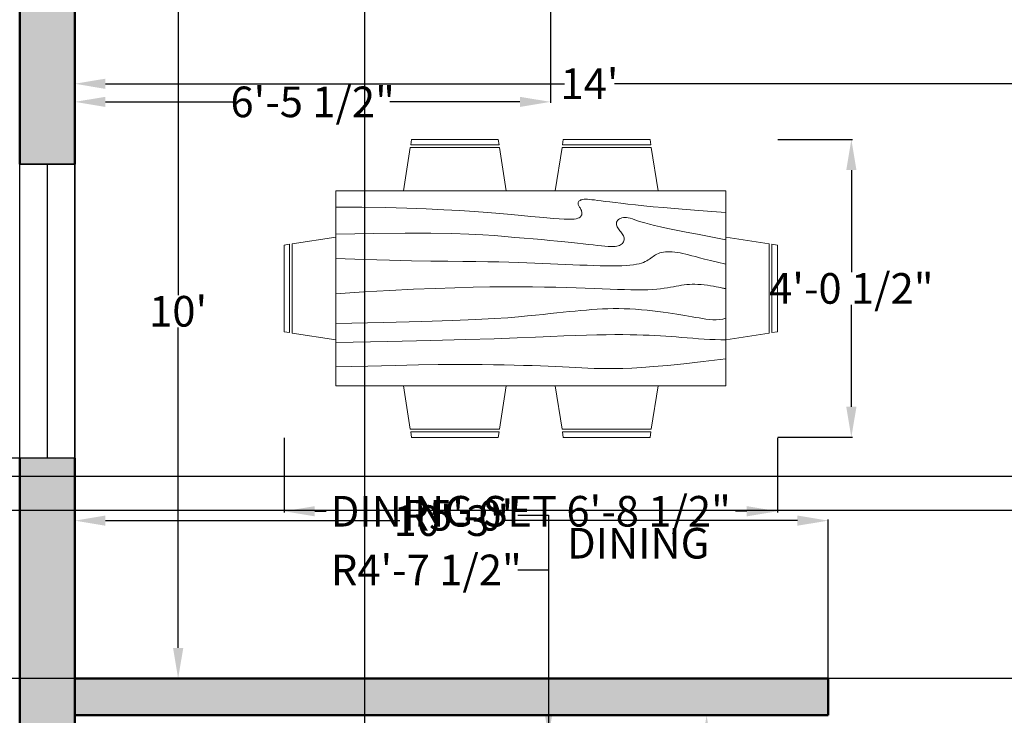
# Model space of a CAD drawing. Units: inches. Extents: x 3136 to 3620, y 13606 to 14152.
# Tile 4 of 6: x 3225 to 3386, y 13852 to 13965. Entities that reach past the tile are written whole.
import ezdxf

# ---------------------------------------------------------------- set-up
doc = ezdxf.new("R2010")
doc.units = ezdxf.units.IN
for name, color, linetype, lineweight in [('A-ANNO-DIMS', 2, 'Continuous', 18), ('A-AREA-IDEN', 7, 'Continuous', 25), ('A-FURN', 8, 'Continuous', 18), ('A-GLAZ', 4, 'Continuous', 25), ('A-WALL', 7, 'Continuous', 50), ('A-WALL-PATT', 174, 'Continuous', 13)]:
    doc.layers.add(name, color=color, linetype=linetype, lineweight=lineweight)
doc.styles.get("Standard").update_dxf_attribs({"font": 'arial.ttf', "height": 5})
doc.dimstyles.get("Standard").update_dxf_attribs({"dimtxt": 5, "dimasz": 5, "dimexe": 0.18, "dimexo": 0.0625, "dimgap": 0.09, "dimtad": 0, "dimtih": 1, "dimtoh": 1, "dimdec": 0, "dimzin": 0, "dimdsep": 46, "dimlunit": 3, "dimtxsty": 'Standard', "dimcen": 0.09, "dimadec": 0, "dimazin": 0, "dimtfac": 1, "dimtdec": 0, "dimtofl": 0, "dimtmove": 0, "dimatfit": 3, "dimfxl": 1, "dimtolj": 1, "dimtzin": 0, "dimarcsym": 0})

# ---------------------------------------------------------------- blocks, each defined once
blk = doc.blocks.new('*D13')
at = {"layer": 'A-ANNO-DIMS', "color": 0, "lineweight": -2, "transparency": 16777216}
for p, q in [((3233.87, 13960.47), (3233.87, 13954.82)), ((3401.87, 13960.47), (3401.87, 13954.82)), ((3238.87, 13955), (3313.77, 13955)), ((3396.87, 13955), (3321.97, 13955))]:
    blk.add_line(p, q, dxfattribs=at)
at = {"layer": 'A-ANNO-DIMS', "color": 0, "transparency": 16777216}
for points in [[(3238.87, 13955.83), (3238.87, 13954.16), (3233.87, 13955)], [(3396.87, 13955.83), (3396.87, 13954.16), (3401.87, 13955)]]:
    blk.add_solid(points, dxfattribs=at)
at = {"layer": 'Defpoints', "color": 0, "transparency": 16777216}
for p in [(3233.87, 13960.54), (3401.87, 13960.54), (3401.87, 13955)]:
    blk.add_point(p, dxfattribs=at)
at = {"layer": 'A-ANNO-DIMS', "color": 0, "transparency": 16777216, "insert": (3317.87, 13955), "char_height": 5, "attachment_point": 5}
blk.add_mtext("\\A1;14'", dxfattribs=at)
blk = doc.blocks.new('*D14')
at = {"layer": 'A-ANNO-DIMS', "color": 0, "lineweight": -2, "transparency": 16777216}
for p, q in [((3233.93, 13977.84), (3250.91, 13977.84)), ((3250.73, 13972.84), (3250.73, 13920.48)), ((3250.73, 13862.84), (3250.73, 13915.2)), ((3233.93, 13857.84), (3250.91, 13857.84))]:
    blk.add_line(p, q, dxfattribs=at)
at = {"layer": 'A-ANNO-DIMS', "color": 0, "transparency": 16777216}
for points in [[(3249.9, 13972.84), (3251.57, 13972.84), (3250.73, 13977.84)], [(3249.9, 13862.84), (3251.57, 13862.84), (3250.73, 13857.84)]]:
    blk.add_solid(points, dxfattribs=at)
at = {"layer": 'Defpoints', "color": 0, "transparency": 16777216}
for p in [(3233.87, 13977.84), (3250.73, 13977.84), (3233.87, 13857.84)]:
    blk.add_point(p, dxfattribs=at)
at = {"layer": 'A-ANNO-DIMS', "color": 0, "transparency": 16777216, "insert": (3250.73, 13917.84), "char_height": 5, "attachment_point": 5}
blk.add_mtext("\\A1;10'", dxfattribs=at)
blk = doc.blocks.new('*D16')
at = {"layer": 'A-ANNO-DIMS', "color": 0, "lineweight": -2, "transparency": 16777216}
for p, q in [((3311.54, 13851.84), (3337.17, 13851.84)), ((3336.99, 13846.84), (3336.99, 13752.44)), ((3336.99, 13652.84), (3336.99, 13747.24)), ((3311.54, 13647.84), (3337.17, 13647.84))]:
    blk.add_line(p, q, dxfattribs=at)
at = {"layer": 'A-ANNO-DIMS', "color": 0, "transparency": 16777216}
for points in [[(3336.16, 13846.84), (3337.82, 13846.84), (3336.99, 13851.84)], [(3336.16, 13652.84), (3337.82, 13652.84), (3336.99, 13647.84)]]:
    blk.add_solid(points, dxfattribs=at)
at = {"layer": 'Defpoints', "color": 0, "transparency": 16777216}
for p in [(3311.47, 13851.84), (3336.99, 13851.84), (3311.47, 13647.84)]:
    blk.add_point(p, dxfattribs=at)
at = {"layer": 'A-ANNO-DIMS', "color": 0, "transparency": 16777216, "insert": (3336.99, 13749.84), "char_height": 5, "attachment_point": 5}
blk.add_mtext("\\A1;17'", dxfattribs=at)
blk = doc.blocks.new('Dining Set - 36 x 72 in.')
for p, q in [((-22, 27.5), (-22.1562, 26.50042)), ((-22, 27.5), (-6, 27.5)), ((-5.8437, 26.49966), (-6, 27.5)), ((6, 27.5), (5.8438, 26.50042)), ((6, 27.5), (22, 27.5)), ((22.1563, 26.49966), (22, 27.5)), ((-22.2343, 26.00059), (-23.4847, 17.99762)), ((-22.2304, 26), (-5.7608, 26)), ((-5.8416, 26.5), (-22.1534, 26.5)), ((-4.5152, 17.99762), (-5.7655, 25.99926)), ((5.7657, 26.00059), (4.5153, 17.99762)), ((5.7696, 26), (22.2392, 26)), ((22.1584, 26.5), (5.8466, 26.5)), ((23.4848, 17.99762), (22.2345, 25.99926)), ((36, 18), (-36, 18)), ((-36, 18), (-36, -18)), ((36, -18), (36, 18)), ((-44.0006, 8.23428), (-35.9976, 9.48474)), ((44.0006, 8.23428), (35.9976, 9.48474)), ((-45.5, 8), (-44.5004, 8.15617)), ((-45.5, 8), (-45.5, -8)), ((-44.5, -8.15843), (-44.5, 8.15338)), ((-44, 8.23041), (-44, -8.23915)), ((44, 8.23041), (44, -8.23915)), ((44.5, -8.15843), (44.5, 8.15338)), ((45.5, 8), (44.5005, 8.15617)), ((45.5, 8), (45.5, -8)), ((-44.4997, -8.15631), (-45.5, -8)), ((-35.9976, -9.48476), (-43.9993, -8.2345)), ((35.9976, -9.48476), (43.9993, -8.2345)), ((44.4997, -8.15631), (45.5, -8)), ((-36, -18), (36, -18)), ((-22.2343, -26.0006), (-23.4847, -17.99762)), ((-4.5152, -17.99762), (-5.7655, -25.99928)), ((5.7657, -26.0006), (4.5153, -17.99762)), ((23.4848, -17.99762), (22.2345, -25.99928)), ((-22.2304, -26), (-5.7608, -26)), ((-22, -27.5), (-22.1562, -26.50044)), ((-5.8416, -26.5), (-22.1534, -26.5)), ((-5.8437, -26.49967), (-6, -27.5)), ((5.7696, -26), (22.2392, -26)), ((6, -27.5), (5.8438, -26.50044)), ((22.1584, -26.5), (5.8466, -26.5)), ((22.1563, -26.49967), (22, -27.5)), ((-22, -27.5), (-6, -27.5)), ((6, -27.5), (22, -27.5))]:
    blk.add_line(p, q)
for points in [[(-36, 15), (-31.1772, 14.97754), (-26.8079, 14.91406), (-22.8538, 14.81543), (-19.276, 14.6875), (-16.0362, 14.53613), (-13.0957, 14.36718), (-10.4159, 14.18652), (-7.9583, 14), (-5.6904, 13.81315), (-3.6035, 13.63021), (-1.6954, 13.45508), (0.0365, 13.29166), (1.5945, 13.14388), (2.9811, 13.01562), (4.1988, 12.9108), (5.25, 12.83333), (6.1393, 12.78613), (6.8802, 12.76823), (7.4883, 12.77767), (7.9792, 12.8125), (8.3685, 12.87077), (8.6719, 12.95052), (8.9049, 13.0498), (9.0833, 13.16666), (9.2205, 13.29899), (9.3216, 13.44401), (9.3895, 13.59879), (9.4271, 13.76041), (9.4373, 13.92594), (9.4232, 14.09245), (9.3875, 14.257), (9.3333, 14.41666), (9.2638, 14.56917), (9.1836, 14.71484), (9.0975, 14.85465), (9.0104, 14.98958), (8.9272, 15.1206), (8.8529, 15.2487), (8.7922, 15.37483), (8.75, 15.5), (8.7305, 15.62467), (8.7344, 15.74739), (8.7617, 15.86621), (8.8125, 15.97916), (8.8867, 16.08431), (8.9844, 16.17968), (9.1055, 16.26334), (9.25, 16.33333), (9.4189, 16.38802), (9.6172, 16.42708), (9.8506, 16.45052), (10.125, 16.45833), (10.4463, 16.45052), (10.8203, 16.42708), (11.2529, 16.38802), (11.75, 16.33333), (12.3184, 16.26318), (12.9694, 16.17838), (13.7151, 16.07991), (14.5677, 15.96875), (15.5395, 15.84586), (16.6426, 15.71224), (17.8893, 15.56884), (19.2917, 15.41666), (20.859, 15.25667), (22.5879, 15.08984), (24.4721, 14.91715), (26.5052, 14.73958), (28.6809, 14.5581), (30.9929, 14.3737), (33.4347, 14.18733), (36, 14)], [(-36, 10), (-28.9766, 10.14274), (-23.1725, 10.20442), (-18.4241, 10.19775), (-14.5677, 10.13541), (-11.4399, 10.03011), (-8.877, 9.89453), (-6.7154, 9.74137), (-4.7917, 9.58333), (-2.9698, 9.43082), (-1.2246, 9.28515), (0.4415, 9.14534), (2.026, 9.01041), (3.5266, 8.87939), (4.9408, 8.7513), (6.266, 8.62516), (7.5, 8.5), (8.6411, 8.37549), (9.6914, 8.2539), (10.6538, 8.13818), (11.5312, 8.03125), (12.3267, 7.93603), (13.043, 7.85547), (13.6831, 7.79248), (14.25, 7.75), (14.7471, 7.7303), (15.1797, 7.73307), (15.5537, 7.75732), (15.875, 7.80208), (16.1494, 7.86637), (16.3828, 7.94922), (16.5811, 8.04964), (16.75, 8.16666), (16.8944, 8.29915), (17.0143, 8.44531), (17.1089, 8.60319), (17.1771, 8.77083), (17.218, 8.94629), (17.2305, 9.1276), (17.2137, 9.31282), (17.1667, 9.5), (17.0895, 9.6875), (16.987, 9.875), (16.8649, 10.0625), (16.7292, 10.25), (16.5856, 10.4375), (16.4401, 10.625), (16.2985, 10.8125), (16.1667, 11), (16.05, 11.18733), (15.9518, 11.3737), (15.8752, 11.5581), (15.8229, 11.73958), (15.798, 11.91715), (15.8034, 12.08984), (15.842, 12.25667), (15.9167, 12.41666), (16.0295, 12.56836), (16.1784, 12.70833), (16.3605, 12.83268), (16.5729, 12.9375), (16.8127, 13.01888), (17.0768, 13.07291), (17.3625, 13.0957), (17.6667, 13.08333), (17.9894, 13.03312), (18.3418, 12.94726), (18.7382, 12.82918), (19.1927, 12.68229), (19.7195, 12.51001), (20.3327, 12.31575), (21.0465, 12.10294), (21.875, 11.875), (22.8357, 11.63354), (23.959, 11.37304), (25.2786, 11.08618), (26.8282, 10.76562), (28.6414, 10.40405), (30.752, 9.99414), (33.1936, 9.52856), (36, 9)], [(-36, 5.5), (-30.7157, 5.3348), (-26.069, 5.20963), (-21.9946, 5.11767), (-18.4271, 5.05208), (-15.3009, 5.00602), (-12.5508, 4.97265), (-10.1112, 4.94515), (-7.9167, 4.91666), (-5.909, 4.88167), (-4.0586, 4.83984), (-2.3429, 4.79215), (-0.7396, 4.73958), (0.7739, 4.6831), (2.22, 4.6237), (3.6213, 4.56233), (5, 4.5), (6.373, 4.43782), (7.7344, 4.3776), (9.0723, 4.32129), (10.375, 4.27083), (11.6309, 4.22819), (12.8281, 4.19531), (13.9551, 4.17415), (15, 4.16666), (15.954, 4.17448), (16.819, 4.19791), (17.6001, 4.23698), (18.3021, 4.29166), (18.9299, 4.36198), (19.4883, 4.44791), (19.9823, 4.54948), (20.4167, 4.66666), (20.7969, 4.79899), (21.1302, 4.94401), (21.4245, 5.09879), (21.6875, 5.26041), (21.9271, 5.42594), (22.1511, 5.59245), (22.3672, 5.757), (22.5834, 5.91666), (22.8065, 6.06868), (23.0404, 6.21093), (23.2879, 6.34147), (23.5521, 6.45833), (23.8358, 6.55957), (24.142, 6.64323), (24.4735, 6.70735), (24.8334, 6.75), (25.2235, 6.76969), (25.642, 6.76692), (26.0858, 6.74267), (26.5521, 6.69791), (27.0379, 6.63362), (27.5404, 6.55078), (28.0565, 6.45036), (28.5834, 6.33333), (29.1242, 6.19987), (29.7071, 6.04687), (30.3661, 5.87044), (31.1354, 5.66666), (32.0493, 5.43164), (33.142, 5.16146), (34.4475, 4.85221), (36, 4.5)], [(-36, -1), (-30.7915, -0.6591), (-26.0195, -0.38216), (-21.6519, -0.16284), (-17.6563, 0.00521), (-14.0005, 0.12833), (-10.6523, 0.21289), (-7.5796, 0.26522), (-4.75, 0.29166), (-2.134, 0.29793), (0.2878, 0.28711), (2.5317, 0.26163), (4.6146, 0.22396), (6.5529, 0.17651), (8.3633, 0.12174), (10.0623, 0.06209), (11.6667, 0), (13.1899, -0.06201), (14.6341, -0.1211), (15.9982, -0.17432), (17.2813, -0.21875), (18.4823, -0.25147), (19.6003, -0.26953), (20.6343, -0.27002), (21.5834, -0.25), (22.4481, -0.20768), (23.2357, -0.14584), (23.9549, -0.06836), (24.6146, 0.02083), (25.2235, 0.11784), (25.7904, 0.21875), (26.3241, 0.31966), (26.8334, 0.41666), (27.3265, 0.50618), (27.8099, 0.58593), (28.2894, 0.65397), (28.7709, 0.70833), (29.2601, 0.74707), (29.763, 0.76823), (30.2855, 0.76985), (30.8334, 0.75), (31.4088, 0.70784), (31.9994, 0.64713), (32.589, 0.57275), (33.1615, 0.48958), (33.7008, 0.4025), (34.1908, 0.3164), (34.6153, 0.23616), (34.9584, 0.16666), (35.2099, 0.11165), (35.3848, 0.07031), (35.504, 0.04069), (35.5886, 0.02083), (35.6594, 0.00879), (35.7377, 0.0026), (35.8442, 0.00032), (36, 0)], [(-36, -6.5), (-27.1843, -6.31267), (-20.084, -6.1263), (-14.469, -5.9419), (-10.1094, -5.76042), (-6.7752, -5.58285), (-4.2363, -5.41016), (-2.2629, -5.24333), (-0.625, -5.08334), (0.8708, -4.93099), (2.2715, -4.78646), (3.5872, -4.64974), (4.8281, -4.52084), (6.0046, -4.39974), (7.127, -4.28646), (8.2053, -4.18099), (9.25, -4.08334), (10.2705, -3.99382), (11.2734, -3.91407), (12.2647, -3.84603), (13.25, -3.79167), (14.2354, -3.75293), (15.2266, -3.73177), (16.2295, -3.73015), (17.25, -3.75), (18.2912, -3.79248), (19.3451, -3.85547), (20.4009, -3.93604), (21.4479, -4.03125), (22.4754, -4.13819), (23.4727, -4.25391), (24.4289, -4.37549), (25.3334, -4.5), (26.1785, -4.62492), (26.9694, -4.74935), (27.7145, -4.87281), (28.4219, -4.99479), (29.1, -5.11483), (29.7572, -5.23242), (30.4016, -5.34709), (31.0417, -5.45834), (31.6837, -5.56437), (32.3262, -5.65821), (32.9658, -5.73153), (33.599, -5.77604), (34.2224, -5.78345), (34.8327, -5.74545), (35.4264, -5.65373), (36, -5.5)], [(-36, -10), (-26.4022, -9.81299), (-18.4675, -9.62891), (-11.9839, -9.45069), (-6.7396, -9.28125), (-2.5226, -9.12354), (0.8789, -8.98047), (3.6769, -8.85498), (6.0833, -8.75), (8.2767, -8.66765), (10.3021, -8.60677), (12.1712, -8.56543), (13.8958, -8.54167), (15.4876, -8.53353), (16.9583, -8.53907), (18.3197, -8.55632), (19.5834, -8.58334), (20.7616, -8.61841), (21.8685, -8.66081), (22.9188, -8.71004), (23.9271, -8.76563), (24.9081, -8.82707), (25.8763, -8.89388), (26.8465, -8.96558), (27.8334, -9.04167), (28.8474, -9.12118), (29.8828, -9.20117), (30.93, -9.27824), (31.9792, -9.34896), (33.0205, -9.40991), (34.0443, -9.45768), (35.0407, -9.48885), (36, -9.5)], [(-36, -14.5), (-30.0881, -14.33513), (-25.0332, -14.21224), (-20.7312, -14.12647), (-17.0781, -14.07292), (-13.97, -14.04671), (-11.3027, -14.04297), (-8.9724, -14.05681), (-6.875, -14.08334), (-4.9224, -14.11833), (-3.0905, -14.16016), (-1.3709, -14.20785), (0.2448, -14.26042), (1.7647, -14.3169), (3.1973, -14.3763), (4.5507, -14.43767), (5.8333, -14.5), (7.0554, -14.5621), (8.235, -14.62175), (9.3922, -14.67652), (10.5469, -14.72396), (11.7192, -14.76164), (12.929, -14.78711), (14.1965, -14.79794), (15.5417, -14.79167), (16.9933, -14.76424), (18.6152, -14.70508), (20.4804, -14.60197), (22.6615, -14.44271), (25.2312, -14.21509), (28.2624, -13.9069), (31.8277, -13.50594), (36, -13)]]:
    blk.add_lwpolyline(points)
blk = doc.blocks.new('*D28')
at = {"layer": 'A-ANNO-DIMS', "color": 0, "lineweight": -2, "transparency": 16777216}
for p, q in [((3224.81, 14118.84), (3200.37, 14118.84)), ((3200.55, 14113.84), (3200.55, 13881.48)), ((3200.55, 13643.84), (3200.55, 13876.2)), ((3224.81, 13638.84), (3200.37, 13638.84))]:
    blk.add_line(p, q, dxfattribs=at)
at = {"layer": 'A-ANNO-DIMS', "color": 0, "transparency": 16777216}
for points in [[(3199.71, 14113.84), (3201.38, 14113.84), (3200.55, 14118.84)], [(3199.71, 13643.84), (3201.38, 13643.84), (3200.55, 13638.84)]]:
    blk.add_solid(points, dxfattribs=at)
at = {"layer": 'Defpoints', "color": 0, "transparency": 16777216}
for p in [(3200.55, 14118.84), (3224.87, 14118.84), (3224.87, 13638.84)]:
    blk.add_point(p, dxfattribs=at)
at = {"layer": 'A-ANNO-DIMS', "color": 0, "transparency": 16777216, "insert": (3200.55, 13878.84), "char_height": 5, "attachment_point": 5}
blk.add_mtext("\\A1;40'", dxfattribs=at)
blk = doc.blocks.new('WIN-48IN-GLAZING')
for p, q in [((0, 0), (0, 9)), ((48, 0), (48, 9)), ((48, 4.5), (0, 4.5))]:
    blk.add_line(p, q)
blk = doc.blocks.new('*D44')
at = {"layer": 'A-ANNO-DIMS', "color": 0, "lineweight": -2, "transparency": 16777216}
for p, q in [((3268.04, 13897.19), (3268.04, 13884.99)), ((3348.54, 13897.19), (3348.54, 13884.99)), ((3273.04, 13885.17), (3274.9, 13885.17)), ((3343.54, 13885.17), (3341.68, 13885.17))]:
    blk.add_line(p, q, dxfattribs=at)
at = {"layer": 'A-ANNO-DIMS', "color": 0, "transparency": 16777216}
for points in [[(3273.04, 13886.01), (3273.04, 13884.34), (3268.04, 13885.17)], [(3343.54, 13886.01), (3343.54, 13884.34), (3348.54, 13885.17)]]:
    blk.add_solid(points, dxfattribs=at)
at = {"layer": 'Defpoints', "color": 0, "transparency": 16777216}
for p in [(3268.04, 13897.25), (3348.54, 13897.25), (3348.54, 13885.17)]:
    blk.add_point(p, dxfattribs=at)
at = {"layer": 'A-ANNO-DIMS', "color": 0, "transparency": 16777216, "insert": (3308.29, 13885.17), "char_height": 5, "attachment_point": 5}
blk.add_mtext('\\A1;DINING SET 6\'-8 1/2"', dxfattribs=at)
blk = doc.blocks.new('*D45')
at = {"layer": 'A-ANNO-DIMS', "color": 0, "lineweight": -2, "transparency": 16777216}
for p, q in [((3348.6, 13945.9), (3360.79, 13945.9)), ((3360.61, 13940.9), (3360.61, 13924.25)), ((3360.61, 13902.25), (3360.61, 13918.9)), ((3348.6, 13897.25), (3360.79, 13897.25))]:
    blk.add_line(p, q, dxfattribs=at)
at = {"layer": 'A-ANNO-DIMS', "color": 0, "transparency": 16777216}
for points in [[(3359.78, 13940.9), (3361.45, 13940.9), (3360.61, 13945.9)], [(3359.78, 13902.25), (3361.45, 13902.25), (3360.61, 13897.25)]]:
    blk.add_solid(points, dxfattribs=at)
at = {"layer": 'Defpoints', "color": 0, "transparency": 16777216}
for p in [(3348.54, 13945.9), (3360.61, 13945.9), (3348.54, 13897.25)]:
    blk.add_point(p, dxfattribs=at)
at = {"layer": 'A-ANNO-DIMS', "color": 0, "transparency": 16777216, "insert": (3360.61, 13921.57), "char_height": 5, "attachment_point": 5}
blk.add_mtext('\\A1;4\'-0 1/2"', dxfattribs=at)
blk = doc.blocks.new('*D49')
at = {"layer": 'A-ANNO-DIMS', "color": 0, "lineweight": -2, "transparency": 16777216}
for p, q in [((3503.81, 13885.32), (3198.89, 13885.32)), ((3199.07, 13880.32), (3199.07, 13874.26)), ((3199.07, 13862.84), (3199.07, 13868.9)), ((3503.81, 13857.84), (3198.89, 13857.84))]:
    blk.add_line(p, q, dxfattribs=at)
at = {"layer": 'A-ANNO-DIMS', "color": 0, "transparency": 16777216}
for points in [[(3198.24, 13880.32), (3199.9, 13880.32), (3199.07, 13885.32)], [(3198.24, 13862.84), (3199.9, 13862.84), (3199.07, 13857.84)]]:
    blk.add_solid(points, dxfattribs=at)
at = {"layer": 'Defpoints', "color": 0, "transparency": 16777216}
for p in [(3199.07, 13885.32), (3503.87, 13885.32), (3503.87, 13857.84)]:
    blk.add_point(p, dxfattribs=at)
at = {"layer": 'A-ANNO-DIMS', "color": 0, "transparency": 16777216, "insert": (3199.07, 13871.58), "char_height": 5, "attachment_point": 5}
blk.add_mtext('\\A1;2\'-3 1/2"', dxfattribs=at)
blk = doc.blocks.new('*D55')
at = {"layer": 'A-ANNO-DIMS', "color": 0, "lineweight": -2, "transparency": 16777216}
for p, q in [((3233.87, 13977.78), (3233.87, 13951.86)), ((3311.51, 13977.78), (3311.51, 13951.86)), ((3238.87, 13952.04), (3260.12, 13952.04)), ((3306.51, 13952.04), (3285.27, 13952.04))]:
    blk.add_line(p, q, dxfattribs=at)
at = {"layer": 'A-ANNO-DIMS', "color": 0, "transparency": 16777216}
for points in [[(3238.87, 13952.87), (3238.87, 13951.21), (3233.87, 13952.04)], [(3306.51, 13952.87), (3306.51, 13951.21), (3311.51, 13952.04)]]:
    blk.add_solid(points, dxfattribs=at)
at = {"layer": 'Defpoints', "color": 0, "transparency": 16777216}
for p in [(3233.87, 13977.84), (3311.51, 13977.84), (3233.87, 13952.04)]:
    blk.add_point(p, dxfattribs=at)
at = {"layer": 'A-ANNO-DIMS', "color": 0, "transparency": 16777216, "insert": (3272.69, 13952.04), "char_height": 5, "attachment_point": 5}
blk.add_mtext('\\A1;6\'-5 1/2"', dxfattribs=at)
blk = doc.blocks.new('*D64')
at = {"layer": 'A-ANNO-DIMS', "color": 0, "lineweight": -2, "transparency": 16777216}
for p, q in [((3233.81, 13893.84), (3207.89, 13893.84)), ((3208.07, 13888.84), (3208.07, 13878.48)), ((3208.07, 13862.84), (3208.07, 13873.19)), ((3233.81, 13857.84), (3207.89, 13857.84))]:
    blk.add_line(p, q, dxfattribs=at)
at = {"layer": 'A-ANNO-DIMS', "color": 0, "transparency": 16777216}
for points in [[(3207.24, 13888.84), (3208.9, 13888.84), (3208.07, 13893.84)], [(3207.24, 13862.84), (3208.9, 13862.84), (3208.07, 13857.84)]]:
    blk.add_solid(points, dxfattribs=at)
at = {"layer": 'Defpoints', "color": 0, "transparency": 16777216}
for p in [(3208.07, 13893.84), (3233.87, 13893.84), (3233.87, 13857.84)]:
    blk.add_point(p, dxfattribs=at)
at = {"layer": 'A-ANNO-DIMS', "color": 0, "transparency": 16777216, "insert": (3208.07, 13875.84), "char_height": 5, "attachment_point": 5}
blk.add_mtext('\\A1;3\'-0"', dxfattribs=at)
blk = doc.blocks.new('*D68')
at = {"layer": 'A-ANNO-DIMS', "color": 0, "lineweight": -2, "transparency": 16777216}
for p, q in [((3233.87, 13857.9), (3233.87, 13883.82)), ((3238.87, 13883.64), (3286.9, 13883.64)), ((3351.82, 13883.64), (3303.79, 13883.64)), ((3356.82, 13857.9), (3356.82, 13883.82))]:
    blk.add_line(p, q, dxfattribs=at)
at = {"layer": 'A-ANNO-DIMS', "color": 0, "transparency": 16777216}
for points in [[(3238.87, 13884.47), (3238.87, 13882.81), (3233.87, 13883.64)], [(3351.82, 13884.47), (3351.82, 13882.81), (3356.82, 13883.64)]]:
    blk.add_solid(points, dxfattribs=at)
at = {"layer": 'Defpoints', "color": 0, "transparency": 16777216}
for p in [(3356.82, 13883.64), (3233.87, 13857.84), (3356.82, 13857.84)]:
    blk.add_point(p, dxfattribs=at)
at = {"layer": 'A-ANNO-DIMS', "color": 0, "transparency": 16777216, "insert": (3295.34, 13883.64), "char_height": 5, "attachment_point": 5}
blk.add_mtext('\\A1;10\'-3"', dxfattribs=at)
blk = doc.blocks.new('*D73')
at = {"layer": 'A-ANNO-DIMS', "color": 0, "lineweight": -2, "transparency": 16777216}
for p, q in [((3551.42, 13890.84), (3198.89, 13890.84)), ((3199.07, 13885.84), (3199.07, 13876.98)), ((3199.07, 13862.84), (3199.07, 13871.7)), ((3540.92, 13857.84), (3198.89, 13857.84))]:
    blk.add_line(p, q, dxfattribs=at)
at = {"layer": 'A-ANNO-DIMS', "color": 0, "transparency": 16777216}
for points in [[(3198.24, 13885.84), (3199.9, 13885.84), (3199.07, 13890.84)], [(3198.24, 13862.84), (3199.9, 13862.84), (3199.07, 13857.84)]]:
    blk.add_solid(points, dxfattribs=at)
at = {"layer": 'Defpoints', "color": 0, "transparency": 16777216}
for p in [(3551.48, 13890.84), (3199.07, 13857.84), (3540.98, 13857.84)]:
    blk.add_point(p, dxfattribs=at)
at = {"layer": 'A-ANNO-DIMS', "color": 0, "transparency": 16777216, "insert": (3199.07, 13874.34), "char_height": 5, "attachment_point": 5}
blk.add_mtext('\\A1;2\'-9"', dxfattribs=at)
blk = doc.blocks.new('*D77')
at = {"layer": 'A-ANNO-DIMS', "color": 0, "lineweight": -2, "transparency": 16777216}
for p, q in [((3233.87, 13851.9), (3233.87, 14144.82)), ((3238.87, 14144.64), (3243.03, 14144.64)), ((3276.19, 14144.64), (3272.03, 14144.64)), ((3281.19, 13814.42), (3281.19, 14144.82))]:
    blk.add_line(p, q, dxfattribs=at)
at = {"layer": 'A-ANNO-DIMS', "color": 0, "transparency": 16777216}
for points in [[(3238.87, 14145.47), (3238.87, 14143.81), (3233.87, 14144.64)], [(3276.19, 14145.47), (3276.19, 14143.81), (3281.19, 14144.64)]]:
    blk.add_solid(points, dxfattribs=at)
at = {"layer": 'Defpoints', "color": 0, "transparency": 16777216}
for p in [(3233.87, 14144.64), (3233.87, 13851.84), (3281.19, 13814.36)]:
    blk.add_point(p, dxfattribs=at)
at = {"layer": 'A-ANNO-DIMS', "color": 0, "transparency": 16777216, "insert": (3257.53, 14144.64), "char_height": 5, "attachment_point": 5}
blk.add_mtext('\\A1;3\'-11 1/2"', dxfattribs=at)
blk = doc.blocks.new('*D80')
at = {"layer": 'A-ANNO-DIMS', "color": 0, "lineweight": -2, "transparency": 16777216}
for p, q in [((3306.19, 13884.51), (3311.19, 13884.51)), ((3311.19, 13884.51), (3311.19, 13853.36)), ((3311.1, 13788.11), (3311.28, 13788.11)), ((3311.19, 13788.02), (3311.19, 13788.2))]:
    blk.add_line(p, q, dxfattribs=at)
at = {"layer": 'A-ANNO-DIMS', "color": 0, "transparency": 16777216}
blk.add_solid([(3312.02, 13853.36), (3310.36, 13853.36), (3311.19, 13848.36)], dxfattribs=at)
at = {"layer": 'Defpoints', "color": 0, "transparency": 16777216}
for p in [(3311.19, 13848.36), (3311.19, 13788.11)]:
    blk.add_point(p, dxfattribs=at)
at = {"layer": 'A-ANNO-DIMS', "color": 0, "transparency": 16777216, "insert": (3297.06, 13884.51), "char_height": 5, "attachment_point": 5}
blk.add_mtext('\\A1;R5\'-0"', dxfattribs=at)
blk = doc.blocks.new('*D81')
at = {"layer": 'A-ANNO-DIMS', "color": 0, "lineweight": -2, "transparency": 16777216}
for p, q in [((3306.19, 13875.59), (3311.19, 13875.59)), ((3311.19, 13875.59), (3311.19, 13847.36)), ((3311.19, 13786.88), (3311.19, 13787.06)), ((3311.1, 13786.97), (3311.28, 13786.97))]:
    blk.add_line(p, q, dxfattribs=at)
at = {"layer": 'A-ANNO-DIMS', "color": 0, "transparency": 16777216}
blk.add_solid([(3312.02, 13847.36), (3310.36, 13847.36), (3311.19, 13842.36)], dxfattribs=at)
at = {"layer": 'Defpoints', "color": 0, "transparency": 16777216}
for p in [(3311.19, 13842.36), (3311.19, 13786.97)]:
    blk.add_point(p, dxfattribs=at)
at = {"layer": 'A-ANNO-DIMS', "color": 0, "transparency": 16777216, "insert": (3291.24, 13875.59), "char_height": 5, "attachment_point": 5}
blk.add_mtext('\\A1;R4\'-7 1/2"', dxfattribs=at)

msp = doc.modelspace()

# ---------------------------------------------------------------- hatches: boundary and pattern name
at = {"layer": 'A-WALL-PATT'}
h = msp.add_hatch(color=256, dxfattribs=at)
h.dxf.hatch_style = 1
h.paths.add_polyline_path([(3584.87, 13767.84), (3575.87, 13767.84), (3575.87, 13714.7), (3584.87, 13714.7)])
h.paths.add_polyline_path([(3584.87, 13666.7), (3575.87, 13666.7), (3575.87, 13647.84), (3398.03, 13647.84), (3398.03, 13638.84), (3584.87, 13638.84)])
h.paths.add_polyline_path([(3350.03, 13647.84), (3272.91, 13647.84, -0.03225), (3273.24, 13642.78), (3273.24, 13638.84), (3350.03, 13638.84)])
h.paths.add_polyline_path([(3233.87, 13724.63), (3224.87, 13724.63), (3224.87, 13638.84), (3233.87, 13638.84), (3233.87, 13642.78), (3233.87, 13682.15)])
h.paths.add_polyline_path([(3233.87, 13893.84), (3224.87, 13893.84), (3224.87, 13760.63), (3233.87, 13760.63)])
h.paths.add_polyline_path([(3356.82, 13857.84), (3233.87, 13857.84), (3233.87, 13851.84), (3356.82, 13851.84)])
h.paths.add_polyline_path([(3233.87, 14022.84), (3224.87, 14022.84), (3224.87, 13941.84), (3233.87, 13941.84)])
h.paths.add_polyline_path([(3311.51, 13983.84), (3233.87, 13983.84), (3233.87, 13977.84), (3311.51, 13977.84)])
h.paths.add_polyline_path([(3467.87, 14118.84), (3224.87, 14118.84), (3224.87, 14070.84), (3233.87, 14070.84), (3233.87, 14081.66), (3233.87, 14109.84), (3467.87, 14109.84)])
h.paths.add_polyline_path([(3575.87, 13935.84), (3435.35, 13935.84, -0.018734), (3435.43, 13933.78), (3435.43, 13929.84), (3575.87, 13929.84)])
h.paths.add_polyline_path([(3417.35, 13932.93), (3424.89, 13932.93), (3424.89, 13943.24), (3417.35, 13943.24)], flags=9)
h.paths.add_polyline_path([(3561.82, 13786.65), (3573.42, 13786.65), (3573.42, 13796.96), (3561.82, 13796.96)], flags=9)
h.paths.add_polyline_path([(3567.12, 13888.65), (3574.84, 13888.65), (3574.84, 13898.96), (3567.12, 13898.96)], flags=9)
h.paths.add_polyline_path([(3536.01, 13916.38), (3543.73, 13916.38), (3543.73, 13926.69), (3536.01, 13926.69)], flags=9)
h.paths.add_polyline_path([(3509.85, 13733.24), (3521.46, 13733.24), (3521.46, 13743.54), (3509.85, 13743.54)], flags=9)
h.paths.add_polyline_path([(3499.97, 13866.95), (3511.39, 13866.95), (3511.39, 13877.25), (3499.97, 13877.25)], flags=9)
h.paths.add_polyline_path([(3456.03, 13744.65), (3463.57, 13744.65), (3463.57, 13754.96), (3456.03, 13754.96)], flags=9)

# ---------------------------------------------------------------- linework, layer by layer
at = {"layer": 'A-GLAZ'}
msp.add_lwpolyline([(3224.87, 13941.84), (3233.87, 13941.84), (3233.87, 13893.84), (3224.87, 13893.84)], close=True, dxfattribs=at)
at = {"layer": 'A-WALL'}
for p, q in [((3233.87, 13941.84), (3233.87, 14022.84)), ((3233.87, 13760.63), (3233.87, 13893.84)), ((3233.87, 13857.84), (3356.82, 13857.84)), ((3356.82, 13851.84), (3356.82, 13857.84)), ((3356.82, 13851.84), (3233.87, 13851.84))]:
    msp.add_line(p, q, dxfattribs=at)
for points in [[(3224.87, 13941.84), (3224.87, 14022.84)], [(3224.87, 13760.63), (3224.87, 13893.84)]]:
    msp.add_lwpolyline(points, dxfattribs=at)

# ---------------------------------------------------------------- block references
at = {"layer": 'A-FURN', "xscale": 0.8845945910985324, "yscale": 0.8845945910985324, "zscale": 0.8845945910985324}
msp.add_blockref('Dining Set - 36 x 72 in.', (3308.29, 13921.57), dxfattribs=at)
at = {"layer": 'A-GLAZ', "rotation": 90.000000000005}
msp.add_blockref('WIN-48IN-GLAZING', (3233.87, 13893.84), dxfattribs=at)

# ---------------------------------------------------------------- texts
at = {"layer": 'A-AREA-IDEN', "insert": (3298.36, 13882.45), "char_height": 5, "attachment_point": 1}
msp.add_mtext_dynamic_manual_height_columns('\\pxqc;DINING', width=54.9344, gutter_width=25, heights=[0], dxfattribs=at)

# ---------------------------------------------------------------- dimensions: what is measured, and where the dimension line sits
at = {"layer": 'A-ANNO-DIMS'}
for base, p1, p2, override, picture, middle in [((3233.87, 14144.64), (3281.19, 13814.36), (3233.87, 13851.84), {"dimdec": 1, "dimlfac": 1, "dimrnd": 0, "dimzin": 1, "dimdsep": 46, "dimlunit": 4, "dimfrac": 2}, '*D77', (3257.53, 14144.64)), ((3401.87, 13955), (3233.87, 13960.54), (3401.87, 13960.54), {"dimclrd": 0, "dimclre": 0, "dimclrt": 0}, '*D13', (3317.87, 13955)), ((3356.8166, 13883.6391), (3233.8713, 13857.8391), (3356.8166, 13857.8391), {"dimdec": 1, "dimlfac": 1, "dimrnd": 0, "dimzin": 1, "dimdsep": 46, "dimlunit": 4, "dimfrac": 2}, '*D68', (3295.3439, 13883.6391))]:
    dim = msp.add_linear_dim(base=base, p1=p1, p2=p2, dimstyle='Standard', override=override, dxfattribs=at)
    dim.commit()
    dim.dimension.update_dxf_attribs({"geometry": picture, "text_midpoint": middle})
for base, p1, p2, angle, override, picture, middle in [((3200.55, 14118.84), (3224.87, 13638.84), (3224.87, 14118.84), 90, {"dimclrd": 0, "dimclre": 0, "dimclrt": 0}, '*D28', (3200.55, 13878.84)), ((3250.73, 13977.84), (3233.87, 13857.84), (3233.87, 13977.84), 90, {"dimclrd": 0, "dimclre": 0, "dimclrt": 0}, '*D14', (3250.73, 13917.84)), ((3233.87, 13952.04), (3311.51, 13977.84), (3233.87, 13977.84), 180, {"dimdec": 1, "dimlfac": 1, "dimrnd": 0, "dimzin": 1, "dimdsep": 46, "dimlunit": 4, "dimfrac": 2}, '*D55', (3272.69, 13952.04)), ((3360.6128, 13945.901), (3348.5381, 13897.2483), (3348.5381, 13945.901), 90, {"dimdec": 1, "dimlfac": 1, "dimrnd": 0, "dimzin": 1, "dimdsep": 46, "dimlunit": 4, "dimfrac": 2}, '*D45', (3360.6128, 13921.5746)), ((3208.07, 13893.84), (3233.87, 13857.84), (3233.87, 13893.84), 90, {"dimdec": 1, "dimlfac": 1, "dimrnd": 0, "dimzin": 1, "dimdsep": 46, "dimlunit": 4, "dimfrac": 2}, '*D64', (3208.07, 13875.84)), ((3199.07, 13857.84), (3551.48, 13890.84), (3540.98, 13857.84), 90, {"dimdec": 1, "dimlfac": 1, "dimrnd": 0, "dimzin": 1, "dimdsep": 46, "dimlunit": 4, "dimfrac": 2}, '*D73', (3199.07, 13874.34)), ((3199.07, 13885.32), (3503.87, 13857.84), (3503.87, 13885.32), 90, {"dimdec": 1, "dimlfac": 1, "dimrnd": 0, "dimzin": 1, "dimdsep": 46, "dimlunit": 4, "dimfrac": 2}, '*D49', (3199.07, 13871.58))]:
    dim = msp.add_linear_dim(base=base, p1=p1, p2=p2, angle=angle, dimstyle='Standard', override=override, dxfattribs=at)
    dim.commit()
    dim.dimension.update_dxf_attribs({"geometry": picture, "text_midpoint": middle})
dim = msp.add_linear_dim(base=(3348.54, 13885.17), p1=(3268.04, 13897.25), p2=(3348.54, 13897.25), text='DINING SET <>', dimstyle='Standard', override={"dimdec": 1, "dimlfac": 1, "dimrnd": 0, "dimzin": 1, "dimdsep": 46, "dimlunit": 4, "dimfrac": 2}, dxfattribs=at)
dim.commit()
dim.dimension.update_dxf_attribs({"geometry": '*D44', "text_midpoint": (3308.29, 13885.17)})
for center, mpoint, picture, middle in [((3311.18914, 13788.1075), (3311.189, 13848.35748), '*D80', (3297.06072, 13884.50746)), ((3311.19, 13786.97), (3311.19, 13842.36), '*D81', (3291.24, 13875.59))]:
    dim = msp.add_radius_dim(center=center, mpoint=mpoint, dimstyle='Standard', override={"dimdec": 1, "dimlfac": 1, "dimrnd": 0, "dimzin": 1, "dimdsep": 46, "dimlunit": 4, "dimfrac": 2}, dxfattribs=at)
    dim.commit()
    dim.dimension.update_dxf_attribs({"geometry": picture, "text_midpoint": middle, "dimtype": 164})
dim = msp.add_linear_dim(base=(3336.99, 13851.84), p1=(3311.47, 13647.84), p2=(3311.47, 13851.84), angle=90, dimstyle='Standard', override={"dimclrd": 0, "dimclre": 0, "dimclrt": 0}, dxfattribs=at)
dim.commit()
dim.dimension.update_dxf_attribs({"geometry": '*D16', "text_midpoint": (3336.99, 13749.84), "dimtype": 160})

doc.saveas('drawing.dxf')
